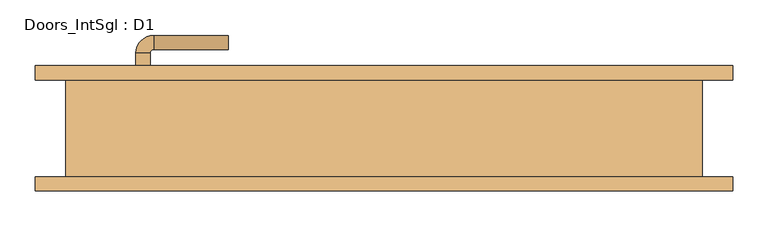
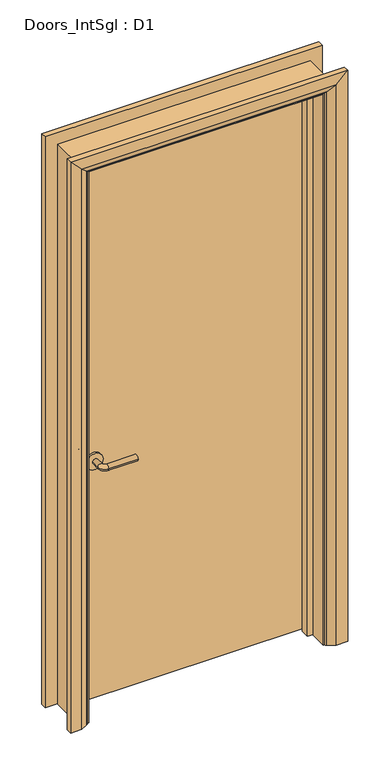
"""IFC4 building model written with IfcOpenShell, lengths in millimetres: door geometry, Doors_IntSgl : D1."""

from ifc_helpers import new_model, si_unit, point, frame, frame_2d, origin, place, context, project, spatial, polyline, circle_curve, ellipse_curve, trimmed, segment, composite_curve, outline, extrude, faceted_brep, source, transform, mapped, element, save
from ifc_brep_helpers import plane_surface, cylinder_surface, revolved_surface, advanced_brep


def doors_intsgl_d1_0ae72840(model_context):
    return source(origin(), model_context, "Body", "SolidModel", [
        advanced_brep(
        [(-350.2, 22.58, 900.0), (-330.2, 22.58, 900.0), (-330.2, -7.42, 900.0), (-350.2, -7.42, 900.0), (-325.2, -12.42, 900.0), (-325.2, -32.42, 900.0), (-220.2, -32.42, 900.0), (-220.2, -12.42, 900.0)],
        [
            (0, 1, circle_curve(frame((-340.2, 22.58, 900.0), z_axis=(0.0, 1.0, 0.0), x_axis=(1.0, 0.0, 0.0)), 10.0)),
            (1, 0, circle_curve(frame((-340.2, 22.58, 900.0), z_axis=(0.0, 1.0, 0.0), x_axis=(1.0, 0.0, 0.0)), 10.0)),
            (1, 2),
            (2, 3, circle_curve(frame((-340.2, -7.42, 900.0), z_axis=(0.0, 1.0, 0.0), x_axis=(1.0, 0.0, 0.0)), 10.0)),
            (3, 0),
            (3, 2, circle_curve(frame((-340.2, -7.42, 900.0), z_axis=(0.0, 1.0, 0.0), x_axis=(1.0, 0.0, 0.0)), 10.0)),
            (4, 5, circle_curve(frame((-325.2, -22.42, 900.0), z_axis=(-1.0, 0.0, 0.0), x_axis=(0.0, 1.0, 0.0)), 10.0)),
            (5, 3, circle_curve(frame((-325.2, -7.42, 900.0), z_axis=(0.0, 0.0, -1.0), x_axis=(-1.0, 0.0, 0.0)), 25.0)),
            (2, 4, circle_curve(frame((-325.2, -7.42, 900.0), z_axis=(0.0, 0.0, 1.0), x_axis=(-1.0, 0.0, 0.0)), 5.0)),
            (5, 4, circle_curve(frame((-325.2, -22.42, 900.0), z_axis=(-1.0, 0.0, 0.0), x_axis=(0.0, 1.0, 0.0)), 10.0)),
            (6, 7, circle_curve(frame((-220.2, -22.42, 900.0), z_axis=(1.0, 0.0, 0.0), x_axis=(0.0, 1.0, 0.0)), 10.0)),
            (7, 6, circle_curve(frame((-220.2, -22.42, 900.0), z_axis=(1.0, 0.0, 0.0), x_axis=(0.0, 1.0, 0.0)), 10.0)),
            (4, 7),
            (6, 5),
        ],
        [
            plane_surface(frame((-340.2, 22.58, 900.0), z_axis=(0.0, 1.0, 0.0), x_axis=(0.0, 0.0, 1.0))),
            cylinder_surface(frame((-340.2, 22.58, 900.0), z_axis=(0.0, 1.0, 0.0), x_axis=(1.0, 0.0, 0.0)), 10.0),
            revolved_surface(trimmed(ellipse_curve(frame((-340.2, -7.42, 900.0), z_axis=(0.0, -1.0, 0.0), x_axis=(1.0, 0.0, 0.0)), 10.0, 10.0), [point((-350.2, -7.42, 900.0))], [point((-330.2, -7.42, 900.0))], True, "CARTESIAN"), (-325.2, -7.42, 900.0), (0.0, 0.0, -1.0)),
            revolved_surface(trimmed(ellipse_curve(frame((-340.2, -7.42, 900.0), z_axis=(0.0, -1.0, 0.0), x_axis=(1.0, 0.0, 0.0)), 10.0, 10.0), [point((-330.2, -7.42, 900.0))], [point((-350.2, -7.42, 900.0))], True, "CARTESIAN"), (-325.2, -7.42, 900.0), (0.0, 0.0, -1.0)),
            plane_surface(frame((-220.2, -22.42, 900.0), z_axis=(1.0, 0.0, 0.0), x_axis=(0.0, 0.0, 1.0))),
            cylinder_surface(frame((-325.2, -22.42, 900.0), z_axis=(-1.0, 0.0, 0.0), x_axis=(0.0, 1.0, 0.0)), 10.0),
        ],
        [
            (0, [[1, 2]]),
            (1, [[3, 4, 5, -2]]),
            (1, [[-5, 6, -3, -1]]),
            (2, [[7, 8, -4, 9]]),
            (3, [[10, -9, -6, -8]]),
            (4, [[11, 12]]),
            (5, [[13, -11, 14, -7]]),
            (5, [[-14, -12, -13, -10]]),
        ],
    ),
        extrude(outline(composite_curve([segment(trimmed(circle_curve(frame_2d((900.0, -342.7)), 30.0), [point((900.0, -372.7))], [point((900.0, -312.7))], False, "CARTESIAN"), True, "CONTINUOUS"), segment(trimmed(circle_curve(frame_2d((900.0, -342.7)), 30.0), [point((900.0, -312.7))], [point((900.0, -372.7))], False, "CARTESIAN"), True, "CONTINUOUS")], self_intersect=False)), frame((0.0, 22.58, 0.0), z_axis=(0.0, 1.0, 0.0), x_axis=(0.0, 0.0, 1.0)), (0.0, 0.0, 1.0), 8.0),
        advanced_brep(
        [(-350.2, 76.58, 900.0), (-330.2, 76.58, 900.0), (-350.2, 106.58, 900.0), (-330.2, 106.58, 900.0), (-325.2, 111.58, 900.0), (-325.2, 131.58, 900.0), (-220.2, 131.58, 900.0), (-220.2, 111.58, 900.0)],
        [
            (0, 1, circle_curve(frame((-340.2, 76.58, 900.0), z_axis=(0.0, -1.0, 0.0), x_axis=(1.0, 0.0, 0.0)), 10.0)),
            (1, 0, circle_curve(frame((-340.2, 76.58, 900.0), z_axis=(0.0, -1.0, 0.0), x_axis=(1.0, 0.0, 0.0)), 10.0)),
            (0, 2),
            (2, 3, circle_curve(frame((-340.2, 106.58, 900.0), z_axis=(0.0, -1.0, 0.0), x_axis=(1.0, 0.0, 0.0)), 10.0)),
            (3, 1),
            (3, 2, circle_curve(frame((-340.2, 106.58, 900.0), z_axis=(0.0, -1.0, 0.0), x_axis=(1.0, 0.0, 0.0)), 10.0)),
            (4, 3, circle_curve(frame((-325.2, 106.58, 900.0), z_axis=(0.0, 0.0, 1.0), x_axis=(-1.0, 0.0, 0.0)), 5.0)),
            (2, 5, circle_curve(frame((-325.2, 106.58, 900.0), z_axis=(0.0, 0.0, -1.0), x_axis=(-1.0, 0.0, 0.0)), 25.0)),
            (5, 4, circle_curve(frame((-325.2, 121.58, 900.0), z_axis=(-1.0, 0.0, 0.0), x_axis=(0.0, -1.0, 0.0)), 10.0)),
            (4, 5, circle_curve(frame((-325.2, 121.58, 900.0), z_axis=(-1.0, 0.0, 0.0), x_axis=(0.0, -1.0, 0.0)), 10.0)),
            (6, 7, circle_curve(frame((-220.2, 121.58, 900.0), z_axis=(1.0, 0.0, 0.0), x_axis=(0.0, -1.0, 0.0)), 10.0)),
            (7, 6, circle_curve(frame((-220.2, 121.58, 900.0), z_axis=(1.0, 0.0, 0.0), x_axis=(0.0, -1.0, 0.0)), 10.0)),
            (5, 6),
            (7, 4),
        ],
        [
            plane_surface(frame((-340.2, 76.58, 900.0), z_axis=(0.0, -1.0, 0.0), x_axis=(0.0, 0.0, 1.0))),
            cylinder_surface(frame((-340.2, 76.58, 900.0), z_axis=(0.0, -1.0, 0.0), x_axis=(1.0, 0.0, 0.0)), 10.0),
            revolved_surface(trimmed(ellipse_curve(frame((-340.2, 106.58, 900.0), z_axis=(0.0, -1.0, 0.0), x_axis=(1.0, 0.0, 0.0)), 10.0, 10.0), [point((-350.2, 106.58, 900.0))], [point((-330.2, 106.58, 900.0))], True, "CARTESIAN"), (-325.2, 106.58, 900.0), (0.0, 0.0, -1.0)),
            revolved_surface(trimmed(ellipse_curve(frame((-340.2, 106.58, 900.0), z_axis=(0.0, -1.0, 0.0), x_axis=(1.0, 0.0, 0.0)), 10.0, 10.0), [point((-330.2, 106.58, 900.0))], [point((-350.2, 106.58, 900.0))], True, "CARTESIAN"), (-325.2, 106.58, 900.0), (0.0, 0.0, -1.0)),
            plane_surface(frame((-220.2, 121.58, 900.0), z_axis=(1.0, 0.0, 0.0), x_axis=(0.0, 0.0, 1.0))),
            cylinder_surface(frame((-325.2, 121.58, 900.0), z_axis=(-1.0, 0.0, 0.0), x_axis=(0.0, -1.0, 0.0)), 10.0),
        ],
        [
            (0, [[1, 2]]),
            (1, [[-1, 3, 4, 5]]),
            (1, [[-2, -5, 6, -3]]),
            (2, [[7, -4, 8, 9]]),
            (3, [[-8, -6, -7, 10]]),
            (4, [[11, 12]]),
            (5, [[-9, 13, -12, 14]]),
            (5, [[-10, -14, -11, -13]]),
        ],
    ),
        extrude(outline(composite_curve([segment(trimmed(circle_curve(frame_2d((900.0, -342.7)), 30.0), [point((900.0, -372.7))], [point((900.0, -312.7))], False, "CARTESIAN"), True, "CONTINUOUS"), segment(trimmed(circle_curve(frame_2d((900.0, -342.7)), 30.0), [point((900.0, -312.7))], [point((900.0, -372.7))], False, "CARTESIAN"), True, "CONTINUOUS")], self_intersect=False)), frame((0.0, 68.58, 0.0), z_axis=(0.0, 1.0, 0.0), x_axis=(0.0, 0.0, 1.0)), (0.0, 0.0, 1.0), 8.0),
        extrude(outline(polyline([(415.2, 30.58), (-415.2, 30.58), (-415.2, 68.58), (415.2, 68.58), (415.2, 30.58)])), frame((0.0, 0.0, 8.0), z_axis=(0.0, 0.0, 1.0), x_axis=(1.0, 0.0, 0.0)), (0.0, 0.0, 1.0), 2060.0),
        advanced_brep(
        [(492.2, 88.58, 0.0), (492.2, 68.58, 0.0), (422.2, 68.58, 0.0), (426.2, 74.58, 0.0), (452.2, 88.58, 0.0), (492.2, 88.58, 2145.0), (492.2, 68.58, 2145.0), (-492.2, 68.58, 2145.0), (-492.2, 68.58, 0.0), (-422.2, 68.58, 0.0), (-422.2, 68.58, 2075.0), (422.2, 68.58, 2075.0), (426.2, 74.58, 2079.0), (452.2, 88.58, 2105.0), (-452.2, 88.58, 2105.0), (-452.2, 88.58, 0.0), (-492.2, 88.58, 0.0), (-492.2, 88.58, 2145.0), (-426.2, 74.58, 0.0), (-426.2, 74.58, 2079.0)],
        [
            (0, 1),
            (1, 2),
            (2, 3, circle_curve(frame((430.2, 67.58, 0.0), z_axis=(0.0, 0.0, -1.0), x_axis=(1.0, 0.0, 0.0)), 8.0622577)),
            (3, 4),
            (4, 0),
            (0, 5),
            (5, 6),
            (6, 1),
            (6, 7),
            (7, 8),
            (8, 9),
            (9, 10),
            (10, 11),
            (11, 2),
            (11, 12, ellipse_curve(frame((430.2, 67.58, 2083.0), z_axis=(0.7071067811865475, 0.0, -0.7071067811865475), x_axis=(-0.7071067811865474, 0.0, -0.7071067811865476)), 11.4017543, 8.0622577)),
            (12, 3),
            (12, 13),
            (13, 4),
            (13, 14),
            (14, 15),
            (15, 16),
            (16, 17),
            (17, 5),
            (7, 17),
            (16, 8),
            (15, 18),
            (18, 9, circle_curve(frame((-430.2, 67.58, 0.0), z_axis=(0.0, 0.0, -1.0), x_axis=(-1.0, 0.0, 0.0)), 8.0622577)),
            (19, 10, ellipse_curve(frame((-430.2, 67.58, 2083.0), z_axis=(-0.7071067811865475, 0.0, -0.7071067811865475), x_axis=(-0.7071067811865474, 0.0, 0.7071067811865476)), 11.4017543, 8.0622577)),
            (18, 19),
            (14, 19),
            (19, 12),
        ],
        [
            plane_surface(frame((422.2, 68.58, 0.0), z_axis=(0.0, 0.0, -1.0), x_axis=(0.0, -1.0, 0.0))),
            plane_surface(frame((492.2, 88.58, 0.0), z_axis=(1.0, 0.0, 0.0), x_axis=(0.0, 0.0, 1.0))),
            plane_surface(frame((492.2, 68.58, 0.0), z_axis=(0.0, -1.0, 0.0), x_axis=(0.0, 0.0, 1.0))),
            cylinder_surface(frame((430.2, 67.58, 0.0), z_axis=(0.0, 0.0, -1.0), x_axis=(1.0, 0.0, 0.0)), 8.0622577),
            plane_surface(frame((426.2, 74.58, 0.0), z_axis=(-0.4740998230350126, 0.880471099922178, 0.0), x_axis=(0.0, 0.0, 1.0))),
            plane_surface(frame((452.2, 88.58, 0.0), z_axis=(0.0, 1.0, 0.0), x_axis=(0.0, 0.0, 1.0))),
            plane_surface(frame((-492.2, 88.58, 2145.0), z_axis=(-1.0, 0.0, 0.0), x_axis=(0.0, 0.0, -1.0))),
            plane_surface(frame((-422.2, 68.58, 0.0), z_axis=(0.0, 0.0, -1.0), x_axis=(0.0, -1.0, 0.0))),
            cylinder_surface(frame((-430.2, 67.58, 2075.0), z_axis=(0.0, 0.0, 1.0), x_axis=(-1.0, 0.0, 0.0)), 8.0622577),
            plane_surface(frame((-426.2, 74.58, 2079.0), z_axis=(0.47409982303501824, 0.8804710999221749, 0.0), x_axis=(0.0, 0.0, -1.0))),
            plane_surface(frame((492.2, 88.58, 2145.0), z_axis=(0.0, 0.0, 1.0), x_axis=(-1.0, 0.0, 0.0))),
            cylinder_surface(frame((422.2, 67.58, 2083.0), z_axis=(1.0, 0.0, 0.0), x_axis=(0.0, 0.0, 1.0)), 8.0622577),
            plane_surface(frame((426.2, 74.58, 2079.0), z_axis=(0.0, 0.8804710999221764, -0.4740998230350154), x_axis=(-1.0, 0.0, 0.0))),
        ],
        [
            (0, [[1, 2, 3, 4, 5]]),
            (1, [[-1, 6, 7, 8]]),
            (2, [[-2, -8, 9, 10, 11, 12, 13, 14]]),
            (3, [[-3, -14, 15, 16]]),
            (4, [[-4, -16, 17, 18]]),
            (5, [[-5, -18, 19, 20, 21, 22, 23, -6]]),
            (6, [[24, -22, 25, -10]]),
            (7, [[-21, 26, 27, -11, -25]]),
            (8, [[28, -12, -27, 29]]),
            (9, [[30, -29, -26, -20]]),
            (10, [[-7, -23, -24, -9]]),
            (11, [[-15, -13, -28, 31]]),
            (12, [[-17, -31, -30, -19]]),
        ],
    ),
        extrude(outline(polyline([(0.0, -417.2), (0.0, -398.2), (2051.0, -398.2), (2051.0, 398.2), (0.0, 398.2), (0.0, 417.2), (2070.0, 417.2), (2070.0, -417.2), (0.0, -417.2)])), frame((0.0, -3.42, 0.0), z_axis=(0.0, 1.0, 0.0), x_axis=(0.0, 0.0, 1.0)), (0.0, 0.0, 1.0), 32.0),
        advanced_brep(
        [(-492.2, -88.58, 0.0), (-492.2, -68.58, 0.0), (-422.2, -68.58, 0.0), (-426.2, -74.58, 0.0), (-452.2, -88.58, 0.0), (-492.2, -88.58, 2145.0), (-492.2, -68.58, 2145.0), (-422.2, -68.58, 2075.0), (-426.2, -74.58, 2079.0), (-452.2, -88.58, 2105.0), (492.2, -88.58, 0.0), (452.2, -88.58, 0.0), (426.2, -74.58, 0.0), (422.2, -68.58, 0.0), (492.2, -68.58, 0.0), (492.2, -88.58, 2145.0), (452.2, -88.58, 2105.0), (426.2, -74.58, 2079.0), (422.2, -68.58, 2075.0), (492.2, -68.58, 2145.0)],
        [
            (0, 1),
            (1, 2),
            (2, 3, circle_curve(frame((-430.2, -67.58, 0.0), z_axis=(0.0, 0.0, -1.0), x_axis=(-1.0, 0.0, 0.0)), 8.0622577)),
            (3, 4),
            (4, 0),
            (0, 5),
            (5, 6),
            (6, 1),
            (6, 7),
            (7, 2),
            (7, 8, ellipse_curve(frame((-430.2, -67.58, 2083.0), z_axis=(-0.7071067811865475, 0.0, -0.7071067811865475), x_axis=(0.7071067811865474, 0.0, -0.7071067811865476)), 11.4017543, 8.0622577)),
            (8, 3),
            (8, 9),
            (9, 4),
            (9, 5),
            (10, 11),
            (11, 12),
            (12, 13, circle_curve(frame((430.2, -67.58, 0.0), z_axis=(0.0, 0.0, -1.0), x_axis=(1.0, 0.0, 0.0)), 8.0622577)),
            (13, 14),
            (14, 10),
            (15, 16),
            (16, 11),
            (10, 15),
            (16, 17),
            (17, 12),
            (17, 18, ellipse_curve(frame((430.2, -67.58, 2083.0), z_axis=(0.7071067811865475, 0.0, -0.7071067811865475), x_axis=(0.7071067811865474, 0.0, 0.7071067811865476)), 11.4017543, 8.0622577)),
            (18, 13),
            (18, 19),
            (19, 14),
            (19, 15),
            (5, 15),
            (19, 6),
            (18, 7),
            (17, 8),
            (16, 9),
        ],
        [
            plane_surface(frame((-422.2, -141.3810989, 0.0), z_axis=(0.0, 0.0, -1.0), x_axis=(1.0, 0.0, 0.0))),
            plane_surface(frame((-492.2, -88.58, 0.0), z_axis=(-1.0, 0.0, 0.0), x_axis=(0.0, 0.0, 1.0))),
            plane_surface(frame((-492.2, -68.58, 0.0), z_axis=(0.0, 1.0, 0.0), x_axis=(0.0, 0.0, 1.0))),
            cylinder_surface(frame((-430.2, -67.58, 0.0), z_axis=(0.0, 0.0, -1.0), x_axis=(-1.0, 0.0, 0.0)), 8.0622577),
            plane_surface(frame((-426.2, -74.58, 0.0), z_axis=(0.4740998230350183, -0.8804710999221749, 0.0), x_axis=(0.0, 0.0, 1.0))),
            plane_surface(frame((-452.2, -88.58, 0.0), z_axis=(0.0, -1.0, 0.0), x_axis=(0.0, 0.0, 1.0))),
            plane_surface(frame((422.2, -141.3810989, 0.0), z_axis=(0.0, 0.0, -1.0), x_axis=(-1.0, 0.0, 0.0))),
            plane_surface(frame((452.2, -88.58, 2105.0), z_axis=(0.0, -1.0, 0.0), x_axis=(0.0, 0.0, -1.0))),
            plane_surface(frame((426.2, -74.58, 2079.0), z_axis=(-0.4740998230350183, -0.8804710999221749, 0.0), x_axis=(0.0, 0.0, -1.0))),
            cylinder_surface(frame((430.2, -67.58, 2075.0), z_axis=(0.0, 0.0, 1.0), x_axis=(1.0, 0.0, 0.0)), 8.0622577),
            plane_surface(frame((492.2, -68.58, 2145.0), z_axis=(0.0, 1.0, 0.0), x_axis=(0.0, 0.0, -1.0))),
            plane_surface(frame((492.2, -88.58, 2145.0), z_axis=(1.0, 0.0, 0.0), x_axis=(0.0, 0.0, -1.0))),
            plane_surface(frame((-492.2, -88.58, 2145.0), z_axis=(0.0, 0.0, 1.0), x_axis=(1.0, 0.0, 0.0))),
            plane_surface(frame((-492.2, -68.58, 2145.0), z_axis=(0.0, 1.0, 0.0), x_axis=(1.0, 0.0, 0.0))),
            cylinder_surface(frame((-422.2, -67.58, 2083.0), z_axis=(-1.0, 0.0, 0.0), x_axis=(0.0, 0.0, 1.0)), 8.0622577),
            plane_surface(frame((-426.2, -74.58, 2079.0), z_axis=(0.0, -0.8804710999221749, -0.4740998230350183), x_axis=(1.0, 0.0, 0.0))),
            plane_surface(frame((-452.2, -88.58, 2105.0), z_axis=(0.0, -1.0, 0.0), x_axis=(1.0, 0.0, 0.0))),
        ],
        [
            (0, [[1, 2, 3, 4, 5]]),
            (1, [[-1, 6, 7, 8]]),
            (2, [[-2, -8, 9, 10]]),
            (3, [[-3, -10, 11, 12]]),
            (4, [[-4, -12, 13, 14]]),
            (5, [[-5, -14, 15, -6]]),
            (6, [[16, 17, 18, 19, 20]]),
            (7, [[21, 22, -16, 23]]),
            (8, [[24, 25, -17, -22]]),
            (9, [[26, 27, -18, -25]]),
            (10, [[28, 29, -19, -27]]),
            (11, [[30, -23, -20, -29]]),
            (12, [[-7, 31, -30, 32]]),
            (13, [[-9, -32, -28, 33]]),
            (14, [[-11, -33, -26, 34]]),
            (15, [[-13, -34, -24, 35]]),
            (16, [[-15, -35, -21, -31]]),
        ],
    ),
        faceted_brep([(-417.2, 68.58, 0.0), (-417.2, -68.58, 0.0), (-449.2, -68.58, 0.0), (-449.2, 68.58, 0.0), (-417.2, 68.58, 2070.0), (-417.2, -68.58, 2070.0), (-449.2, -68.58, 2102.0), (-449.2, 68.58, 2102.0), (417.2, 68.58, 0.0), (449.2, 68.58, 0.0), (449.2, -68.58, 0.0), (417.2, -68.58, 0.0), (417.2, 68.58, 2070.0), (449.2, 68.58, 2102.0), (449.2, -68.58, 2102.0), (417.2, -68.58, 2070.0)], [[[0, 1, 2, 3]], [[1, 0, 4, 5]], [[2, 1, 5, 6]], [[3, 2, 6, 7]], [[0, 3, 7, 4]], [[8, 9, 10, 11]], [[12, 13, 9, 8]], [[13, 14, 10, 9]], [[14, 15, 11, 10]], [[15, 12, 8, 11]], [[5, 4, 12, 15]], [[6, 5, 15, 14]], [[7, 6, 14, 13]], [[4, 7, 13, 12]]]),
    ])


if __name__ == "__main__":
    model = new_model("IFC4")
    model_context = context("Model", 3, world=origin())
    ifc_project = project(units=[si_unit("LENGTHUNIT", "METRE", prefix="MILLI")], contexts=[model_context])
    site = spatial("IfcSite", under=ifc_project)
    building = spatial("IfcBuilding", under=site)
    placement = place(None, origin())
    doors_intsgl_d1_shape = doors_intsgl_d1_0ae72840(model_context)
    element("IfcDoor", 1, ObjectType="Doors_IntSgl : D1", at=placement, inside=building, context=model_context, shape_type="MappedRepresentation", body=[
        mapped(doors_intsgl_d1_shape, transform((0.0, 0.0, 0.0), x_axis=(1.0, 0.0, 0.0), y_axis=(0.0, 1.0, 0.0), z_axis=(0.0, 0.0, 1.0))),
    ])
    save(model, "model.ifc")

# Revit data of these elements
# Type "Doors_IntSgl : D1"
#   Type Mark = "46"
#   Type Comments = "Internal Single"
#   Operation = "SingleSwingRight"
#   Manufacturer = "Revit"
#   Keynote = "L20"
#   Description = "Internal Single Door"
#   Analytic Construction = "Metal"
#   UnderCut = 0.026247 ft
#   Tolerance = 0.006562 ft
#   Thickness = 0.124672 ft
#   Thermal Resistance (R) = 0.270117 (m²·K)/W
#   Structural Tolerance = 0.026247 ft
#   StopDepth = 0.104987 ft
#   Stop Thickness = 0.062336 ft
#   Rough Width = 3.0 ft
#   Rough Height = 6.922572 ft
#   Height to Top Lock Rail = 3.28084 ft
#   Heat Transfer Coefficient (U) = 3.7021 W/(m²·K)
#   Handle Z Distance = 2.952756 ft
#   Handle X Distance = 0.246063 ft
#   Frame Thickness = 0.104987 ft
#   Door Panel Width = 2.724409 ft
#   Door Panel Thickness = 0.124672 ft
#   Door Panel Offset = 0.0 ft
#   Height = 6.922572 ft
#   Width = 3.0 ft
#   Door Panel Height = 6.75853 ft
#   Architrave Setback = 0.016404 ft
#   Vis - Ironmongery = yes
#   Material Ironmongery = Door - Handle
#   Material Frame = Door - Frame/Mullion (1)
#   Material Door = Door - Panel
#   Material Architrave = Door - Architrave
#   Visual Light Transmittance = 0
#   Solar Heat Gain Coefficient = 0
#   Function = (empty or 0)
#   Wall Closure = (empty or 0)
# Element 1 (IfcDoor, "Doors_IntSgl : D1")
#   Materials on its faces: "Door - Architrave", "Door - Handle", "Door - Frame/Mullion (1)", "Door - Panel"
# Materials
#   "Door - Handle": colour RGB 0 0 0, transparency 0, Keynote = "P21", Cost = 0
#   "Door - Frame/Mullion (1)": class "Wood", colour RGB 212 179 113, transparency 0, Keynote = "L20", Cost = 0
#   "Door - Panel": class "Wood", colour RGB 210 159 95, transparency 0, Keynote = "L20", Cost = 0
#   "Door - Architrave": class "Wood", colour RGB 154 90 5, transparency 0, Keynote = "P20", Cost = 0
